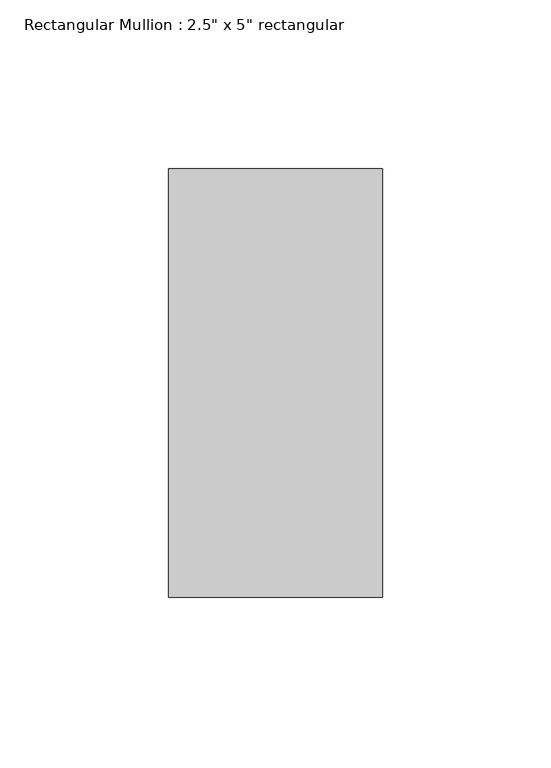
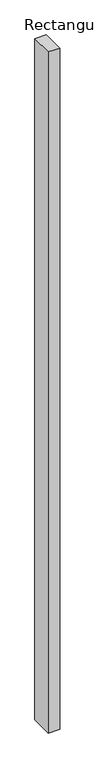
"""IFC4 building model written with IfcOpenShell, lengths in millimetres: member geometry."""

from ifc_helpers import new_model, si_unit, frame, origin, place, context, project, spatial, polyline, outline, extrude, source, transform, mapped, element, save


def member_97fca31a(model_context):
    return source(origin(), model_context, "Body", "SweptSolid", [
        extrude(outline(polyline([(0.0, 63.5), (0.0, -63.5), (-63.5, -63.5), (-63.5, 63.5), (0.0, 63.5)])), frame((0.0, 0.0, -3979.3994026), z_axis=(0.0, 0.0, 1.0), x_axis=(1.0, 0.0, 0.0)), (0.0, 0.0, 1.0), 3979.3994026),
    ])


if __name__ == "__main__":
    model = new_model("IFC4")
    model_context = context("Model", 3, world=origin())
    ifc_project = project(units=[si_unit("LENGTHUNIT", "METRE", prefix="MILLI")], contexts=[model_context])
    site = spatial("IfcSite", under=ifc_project)
    building = spatial("IfcBuilding", under=site)
    placement = place(None, origin())
    member_shape = member_97fca31a(model_context)
    element("IfcMember", 1, ObjectType="Rectangular Mullion : 2.5\" x 5\" rectangular", at=placement, inside=building, context=model_context, shape_type="MappedRepresentation", body=[
        mapped(member_shape, transform((0.0, 0.0, 0.0), x_axis=(1.0, 0.0, 0.0), y_axis=(0.0, 1.0, 0.0), z_axis=(0.0, 0.0, 1.0))),
    ])
    save(model, "model.ifc")

# Revit data of these elements
# Type "Rectangular Mullion : 2.5\" x 5\" rectangular"
#   built-in parameter 1007304 = 0.416667 (stored number, unit not read)
#   built-in parameter 1007301 = 0.104167 (stored number, unit not read)
#   built-in parameter 1007300 = 0.104167 (stored number, unit not read)
# Element 1 (IfcMember, "Rectangular Mullion : 2.5\" x 5\" rectangular")
#   Materials on its faces: "Aluminum"
# Materials
#   "Aluminum": class "Metal", colour RGB 247 247 247, transparency 0, Description = "Aluminum 6061", Cost = 0
